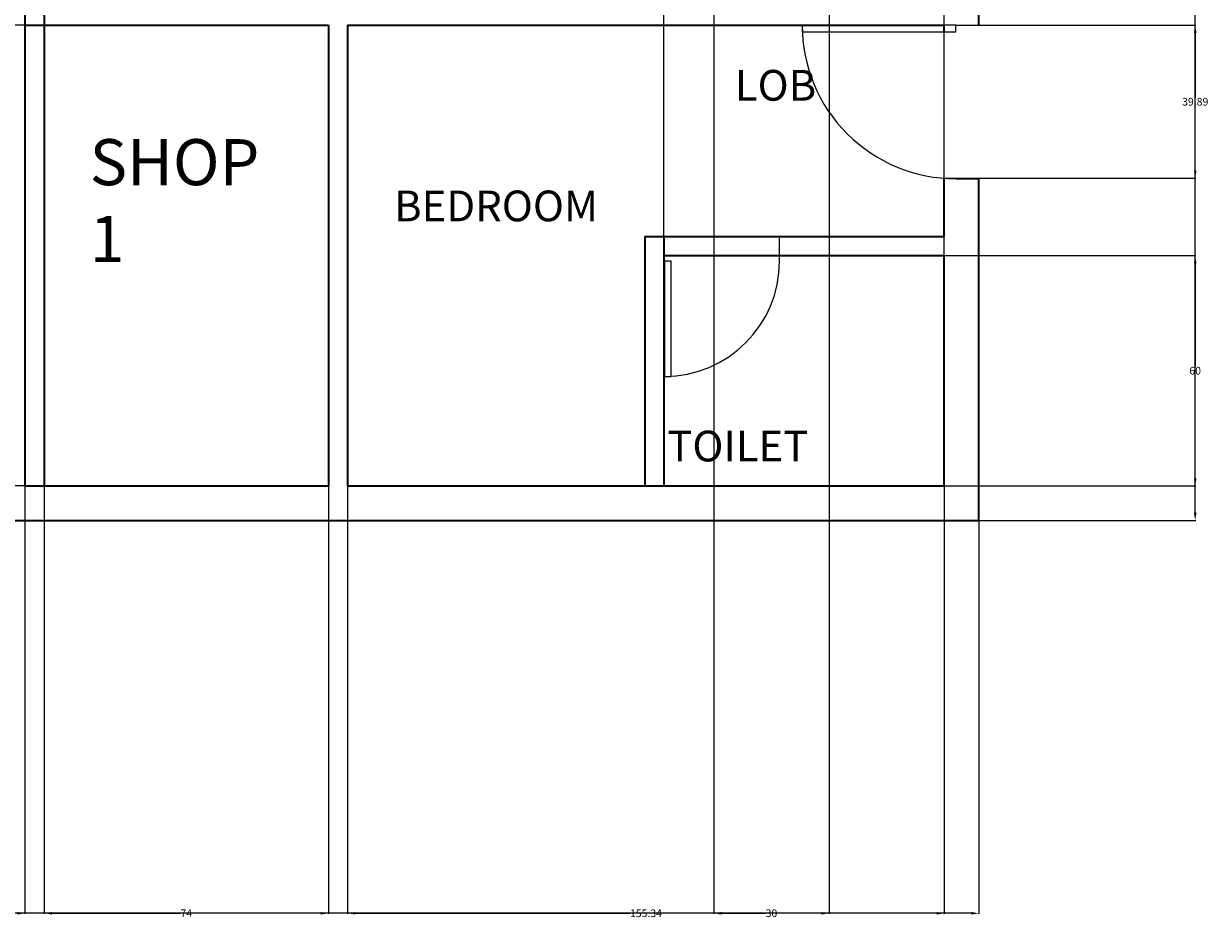
# Model space of a CAD drawing. Units: inches. Extents: x 190 to 836, y -241 to 999.
# Tile 3 of 9: x 528 to 836, y -241 to -8. Entities that reach past the tile are written whole.
import ezdxf

# ---------------------------------------------------------------- set-up
doc = ezdxf.new("R2010")
doc.units = ezdxf.units.IN
doc.header["$MEASUREMENT"] = 0
for name, color, linetype, lineweight in [('A-ANNO-DIMS', 2, 'Continuous', 18), ('A-AREA-IDEN', 7, 'Continuous', 18), ('A-DOOR', 3, 'Continuous', 18), ('A-WALL', 7, 'Continuous', 35)]:
    doc.layers.add(name, color=color, linetype=linetype, lineweight=lineweight)
doc.styles.get("Standard").update_dxf_attribs({"font": 'arial.ttf'})
doc.dimstyles.get("Standard").update_dxf_attribs({"dimtxt": 2, "dimasz": 2, "dimexe": 0.18, "dimexo": 0.0625, "dimgap": 0.09, "dimtad": 0, "dimtih": 1, "dimtoh": 1, "dimdec": 0, "dimzin": 0, "dimdsep": 46, "dimlunit": 3, "dimtxsty": 'Standard', "dimcen": 0.09, "dimadec": 0, "dimazin": 0, "dimtfac": 1, "dimtdec": 0, "dimtofl": 0, "dimtmove": 0, "dimatfit": 3, "dimfxl": 1, "dimtolj": 1, "dimtzin": 0, "dimarcsym": 0})

# ---------------------------------------------------------------- blocks, each defined once
blk = doc.blocks.new('*U3')
for p, q in [((-30, 0), (-30, -6)), ((0, 0), (0, -6))]:
    blk.add_line(p, q)
blk.add_lwpolyline([(0, 0), (0, 30), (-1.75, 30), (-1.75, 0)], close=True)
blk.add_arc((0, 0), 30, 90, 180)
blk = doc.blocks.new('*U2')
for p, q in [((0, 0), (0, 6)), ((40, 0), (40, 6))]:
    blk.add_line(p, q)
blk.add_lwpolyline([(0, 0), (0, -40), (1.75, -40), (1.75, 0)], close=True)
blk.add_arc((0, 0), 40, 270, 360)
blk = doc.blocks.new('*D16')
at = {"layer": 'A-ANNO-DIMS', "color": 0, "lineweight": -2, "transparency": 16777216}
for p, q in [((250.44, -137.53), (250.44, -239.95)), ((776.44, -137.53), (776.44, -239.95)), ((252.44, -239.77), (511.14, -239.77)), ((774.44, -239.77), (515.74, -239.77))]:
    blk.add_line(p, q, dxfattribs=at)
at = {"layer": 'A-ANNO-DIMS', "color": 0, "transparency": 16777216}
for points in [[(252.44, -239.44), (252.44, -240.11), (250.44, -239.77)], [(774.44, -239.44), (774.44, -240.11), (776.44, -239.77)]]:
    blk.add_solid(points, dxfattribs=at)
at = {"layer": 'Defpoints', "color": 0, "transparency": 16777216}
for p in [(250.44, -137.47), (776.44, -137.47), (776.44, -239.77)]:
    blk.add_point(p, dxfattribs=at)
at = {"layer": 'A-ANNO-DIMS', "color": 0, "transparency": 16777216, "insert": (513.44, -239.77), "char_height": 2, "attachment_point": 5}
blk.add_mtext('\\A1;526', dxfattribs=at)
blk = doc.blocks.new('*D18')
at = {"layer": 'A-ANNO-DIMS', "color": 0, "lineweight": -2, "transparency": 16777216}
for p, q in [((776.5, 941.53), (832.94, 941.53)), ((832.76, 939.53), (832.76, 403.14)), ((832.76, -135.47), (832.76, 400.92)), ((776.5, -137.47), (832.94, -137.47))]:
    blk.add_line(p, q, dxfattribs=at)
at = {"layer": 'A-ANNO-DIMS', "color": 0, "transparency": 16777216}
for points in [[(832.43, 939.53), (833.1, 939.53), (832.76, 941.53)], [(832.43, -135.47), (833.1, -135.47), (832.76, -137.47)]]:
    blk.add_solid(points, dxfattribs=at)
at = {"layer": 'Defpoints', "color": 0, "transparency": 16777216}
for p in [(776.44, 941.53), (832.76, 941.53), (776.44, -137.47)]:
    blk.add_point(p, dxfattribs=at)
at = {"layer": 'A-ANNO-DIMS', "color": 0, "transparency": 16777216, "insert": (832.76, 402.03), "char_height": 2, "attachment_point": 5}
blk.add_mtext('\\A1;1079', dxfattribs=at)
blk = doc.blocks.new('*D31')
at = {"layer": 'A-ANNO-DIMS', "color": 0, "lineweight": -2, "transparency": 16777216}
for p, q in [((707.44, 855.47), (707.44, -239.95)), ((737.44, 855.47), (737.44, -239.95)), ((709.44, -239.77), (720.92, -239.77)), ((735.44, -239.77), (723.96, -239.77))]:
    blk.add_line(p, q, dxfattribs=at)
at = {"layer": 'A-ANNO-DIMS', "color": 0, "transparency": 16777216}
for points in [[(709.44, -239.44), (709.44, -240.11), (707.44, -239.77)], [(735.44, -239.44), (735.44, -240.11), (737.44, -239.77)]]:
    blk.add_solid(points, dxfattribs=at)
at = {"layer": 'Defpoints', "color": 0, "transparency": 16777216}
for p in [(707.44, 855.53), (737.44, 855.53), (707.44, -239.77)]:
    blk.add_point(p, dxfattribs=at)
at = {"layer": 'A-ANNO-DIMS', "color": 0, "transparency": 16777216, "insert": (722.44, -239.77), "char_height": 2, "attachment_point": 5}
blk.add_mtext('\\A1;30', dxfattribs=at)
blk = doc.blocks.new('*D37')
at = {"layer": 'A-ANNO-DIMS', "color": 0, "lineweight": -2, "transparency": 16777216}
for p, q in [((528.1, -128.53), (528.1, -239.95)), ((447.44, -137.53), (447.44, -239.95)), ((449.44, -239.77), (484.31, -239.77)), ((526.1, -239.77), (491.24, -239.77))]:
    blk.add_line(p, q, dxfattribs=at)
at = {"layer": 'A-ANNO-DIMS', "color": 0, "transparency": 16777216}
for points in [[(449.44, -239.44), (449.44, -240.11), (447.44, -239.77)], [(526.1, -239.44), (526.1, -240.11), (528.1, -239.77)]]:
    blk.add_solid(points, dxfattribs=at)
at = {"layer": 'Defpoints', "color": 0, "transparency": 16777216}
for p in [(528.1, -128.47), (447.44, -137.47), (528.1, -239.77)]:
    blk.add_point(p, dxfattribs=at)
at = {"layer": 'A-ANNO-DIMS', "color": 0, "transparency": 16777216, "insert": (487.77, -239.77), "char_height": 2, "attachment_point": 5}
blk.add_mtext('\\A1;80.66', dxfattribs=at)
blk = doc.blocks.new('*D38')
at = {"layer": 'A-ANNO-DIMS', "color": 0, "lineweight": -2, "transparency": 16777216}
for p, q in [((533.1, -128.53), (533.1, -239.95)), ((607.1, -128.53), (607.1, -239.95)), ((535.1, -239.77), (568.59, -239.77)), ((605.1, -239.77), (571.61, -239.77))]:
    blk.add_line(p, q, dxfattribs=at)
at = {"layer": 'A-ANNO-DIMS', "color": 0, "transparency": 16777216}
for points in [[(535.1, -239.44), (535.1, -240.11), (533.1, -239.77)], [(605.1, -239.44), (605.1, -240.11), (607.1, -239.77)]]:
    blk.add_solid(points, dxfattribs=at)
at = {"layer": 'Defpoints', "color": 0, "transparency": 16777216}
for p in [(533.1, -128.47), (607.1, -128.47), (607.1, -239.77)]:
    blk.add_point(p, dxfattribs=at)
at = {"layer": 'A-ANNO-DIMS', "color": 0, "transparency": 16777216, "insert": (570.1, -239.77), "char_height": 2, "attachment_point": 5}
blk.add_mtext('\\A1;74', dxfattribs=at)
blk = doc.blocks.new('*D39')
at = {"layer": 'A-ANNO-DIMS', "color": 0, "lineweight": -2, "transparency": 16777216}
for p, q in [((612.1, -128.53), (612.1, -239.95)), ((767.44, -128.53), (767.44, -239.95)), ((614.1, -239.77), (685.63, -239.77)), ((765.44, -239.77), (693.91, -239.77))]:
    blk.add_line(p, q, dxfattribs=at)
at = {"layer": 'A-ANNO-DIMS', "color": 0, "transparency": 16777216}
for points in [[(614.1, -239.44), (614.1, -240.11), (612.1, -239.77)], [(765.44, -239.44), (765.44, -240.11), (767.44, -239.77)]]:
    blk.add_solid(points, dxfattribs=at)
at = {"layer": 'Defpoints', "color": 0, "transparency": 16777216}
for p in [(612.1, -128.47), (767.44, -128.47), (767.44, -239.77)]:
    blk.add_point(p, dxfattribs=at)
at = {"layer": 'A-ANNO-DIMS', "color": 0, "transparency": 16777216, "insert": (689.77, -239.77), "char_height": 2, "attachment_point": 5}
blk.add_mtext('\\A1;155.34', dxfattribs=at)
blk = doc.blocks.new('*D40')
at = {"layer": 'A-ANNO-DIMS', "color": 0, "lineweight": -2, "transparency": 16777216}
for p, q in [((528.04, -8.47), (193.96, -8.47)), ((194.14, -10.47), (194.14, -67.36)), ((194.14, -126.47), (194.14, -69.58)), ((533.04, -128.47), (193.96, -128.47))]:
    blk.add_line(p, q, dxfattribs=at)
at = {"layer": 'A-ANNO-DIMS', "color": 0, "transparency": 16777216}
for points in [[(193.8, -10.47), (194.47, -10.47), (194.14, -8.47)], [(193.8, -126.47), (194.47, -126.47), (194.14, -128.47)]]:
    blk.add_solid(points, dxfattribs=at)
at = {"layer": 'Defpoints', "color": 0, "transparency": 16777216}
for p in [(194.14, -8.47), (528.1, -8.47), (533.1, -128.47)]:
    blk.add_point(p, dxfattribs=at)
at = {"layer": 'A-ANNO-DIMS', "color": 0, "transparency": 16777216, "insert": (194.14, -68.47), "char_height": 2, "attachment_point": 5}
blk.add_mtext('\\A1;120', dxfattribs=at)
blk = doc.blocks.new('*D43')
at = {"layer": 'A-ANNO-DIMS', "color": 0, "lineweight": -2, "transparency": 16777216}
for p, q in [((694.44, -128.41), (694.44, 998.02)), ((696.44, 997.84), (729.43, 997.84)), ((765.44, 997.84), (732.45, 997.84)), ((767.44, -128.41), (767.44, 998.02))]:
    blk.add_line(p, q, dxfattribs=at)
at = {"layer": 'A-ANNO-DIMS', "color": 0, "transparency": 16777216}
for points in [[(696.44, 998.17), (696.44, 997.5), (694.44, 997.84)], [(765.44, 998.17), (765.44, 997.5), (767.44, 997.84)]]:
    blk.add_solid(points, dxfattribs=at)
at = {"layer": 'Defpoints', "color": 0, "transparency": 16777216}
for p in [(767.44, 997.84), (694.44, -128.47), (767.44, -128.47)]:
    blk.add_point(p, dxfattribs=at)
at = {"layer": 'A-ANNO-DIMS', "color": 0, "transparency": 16777216, "insert": (730.94, 997.84), "char_height": 2, "attachment_point": 5}
blk.add_mtext('\\A1;73', dxfattribs=at)
blk = doc.blocks.new('*D44')
at = {"layer": 'A-ANNO-DIMS', "color": 0, "lineweight": -2, "transparency": 16777216}
for p, q in [((767.5, -68.47), (832.94, -68.47)), ((832.76, -70.47), (832.76, -97.36)), ((832.76, -126.47), (832.76, -99.58)), ((767.5, -128.47), (832.94, -128.47))]:
    blk.add_line(p, q, dxfattribs=at)
at = {"layer": 'A-ANNO-DIMS', "color": 0, "transparency": 16777216}
for points in [[(832.43, -70.47), (833.1, -70.47), (832.76, -68.47)], [(832.43, -126.47), (833.1, -126.47), (832.76, -128.47)]]:
    blk.add_solid(points, dxfattribs=at)
at = {"layer": 'Defpoints', "color": 0, "transparency": 16777216}
for p in [(767.44, -68.47), (832.76, -68.47), (767.44, -128.47)]:
    blk.add_point(p, dxfattribs=at)
at = {"layer": 'A-ANNO-DIMS', "color": 0, "transparency": 16777216, "insert": (832.76, -98.47), "char_height": 2, "attachment_point": 5}
blk.add_mtext('\\A1;60', dxfattribs=at)
blk = doc.blocks.new('*D48')
at = {"layer": 'A-ANNO-DIMS', "color": 0, "lineweight": -2, "transparency": 16777216}
for p, q in [((776.5, -8.47), (832.94, -8.47)), ((832.76, -10.47), (832.76, -27.3)), ((832.76, -46.36), (832.76, -29.52)), ((767.5, -48.36), (832.94, -48.36))]:
    blk.add_line(p, q, dxfattribs=at)
at = {"layer": 'A-ANNO-DIMS', "color": 0, "transparency": 16777216}
for points in [[(832.43, -10.47), (833.1, -10.47), (832.76, -8.47)], [(832.43, -46.36), (833.1, -46.36), (832.76, -48.36)]]:
    blk.add_solid(points, dxfattribs=at)
at = {"layer": 'Defpoints', "color": 0, "transparency": 16777216}
for p in [(776.44, -8.47), (832.76, -8.47), (767.44, -48.36)]:
    blk.add_point(p, dxfattribs=at)
at = {"layer": 'A-ANNO-DIMS', "color": 0, "transparency": 16777216, "insert": (832.76, -28.41), "char_height": 2, "attachment_point": 5}
blk.add_mtext('\\A1;39.89', dxfattribs=at)

msp = doc.modelspace()

# ---------------------------------------------------------------- linework, layer by layer
at = {"layer": 'A-WALL'}
for p, q in [((776.4421, -8.4687), (776.4421, 565.5313)), ((528.0998, 115.5313), (528.0998, -128.4687)), ((533.0998, 115.5313), (533.0998, -128.4687)), ((528.0998, -8.4687), (607.0998, -8.4687)), ((607.0998, -8.4687), (607.0998, -128.4687)), ((612.0998, -8.4687), (767.4421, -8.4687)), ((612.0998, -8.4687), (612.0998, -128.4687)), ((767.4421, -10.2187), (767.4421, -8.4687)), ((767.4421, -10.2187), (767.4421, -8.4687)), ((767.4421, -63.4687), (767.4421, -48.356)), ((767.4421, -63.4687), (767.4421, -48.356)), ((776.4421, -137.4687), (776.4421, -48.4687)), ((689.4376, -63.4687), (689.4376, -128.4687)), ((689.4376, -63.4687), (767.4421, -63.4687)), ((694.4376, -68.4687), (694.4376, -128.4687)), ((694.4376, -68.4687), (767.4421, -68.4687)), ((767.4421, -128.4687), (767.4421, -68.4687)), ((767.4421, -128.4687), (767.4421, -68.4687)), ((528.0998, -128.4687), (607.0998, -128.4687)), ((528.0998, -128.4687), (607.0998, -128.4687)), ((612.0998, -128.4687), (672.0998, -128.4687)), ((612.0998, -128.4687), (767.4421, -128.4687)), ((677.0998, -128.4687), (767.4421, -128.4687)), ((499.4421, -137.4687), (776.4421, -137.4687))]:
    msp.add_line(p, q, dxfattribs=at)

# ---------------------------------------------------------------- block references
at = {"layer": 'A-DOOR'}
for name, p, rotation in [('*U2', (770.4421, -8.4687), 269.9999999999999), ('*U3', (694.5596, -69.9458), 179.9999999999999)]:
    msp.add_blockref(name, p, dxfattribs=dict(at, rotation=rotation))

# ---------------------------------------------------------------- texts
at = {"layer": 'A-AREA-IDEN'}
for s, width, insert, char_height, attachment_point in [('LOB', 33.040256, (734.1, -28.136), 8, 9), ('SHOP 1', 18.36577, (544.9435, -38.1547), 12, 1), ('BEDROOM', 33.040256, (677.2999, -59.5532), 8, 9), ('TOILET', 33.040256, (732.0386, -122.0908), 8, 9)]:
    msp.add_mtext_dynamic_manual_height_columns(s, width=width, gutter_width=1, heights=[0], dxfattribs=dict(at, insert=insert, char_height=char_height, attachment_point=attachment_point))

# ---------------------------------------------------------------- dimensions: what is measured, and where the dimension line sits
at = {"layer": 'A-ANNO-DIMS'}
for base, p1, p2, override, picture, middle in [((767.4421, 997.8363), (694.4376, -128.4687), (767.4421, -128.4687), {"dimdec": 0, "dimlfac": 1, "dimrnd": 0, "dimzin": 0, "dimdsep": 46, "dimlunit": 2}, '*D43', (730.9399, 997.8363)), ((707.4421, -239.7737), (737.4421, 855.5313), (707.4421, 855.5313), {"dimdec": 0, "dimlfac": 1, "dimrnd": 0, "dimzin": 0, "dimdsep": 46, "dimlunit": 2}, '*D31', (722.4421, -239.7737)), ((528.0998, -239.7737), (447.4421, -137.4687), (528.0998, -128.4687), {"dimdec": 2, "dimlfac": 1, "dimrnd": 0, "dimzin": 0, "dimdsep": 46, "dimlunit": 2}, '*D37', (487.771, -239.7737)), ((607.0998, -239.7737), (533.0998, -128.4687), (607.0998, -128.4687), {"dimdec": 0, "dimlfac": 1, "dimrnd": 0, "dimzin": 0, "dimdsep": 46, "dimlunit": 2}, '*D38', (570.0998, -239.7737)), ((767.4421, -239.7737), (612.0998, -128.4687), (767.4421, -128.4687), {"dimdec": 2, "dimlfac": 1, "dimrnd": 0, "dimzin": 0, "dimdsep": 46, "dimlunit": 2}, '*D39', (689.771, -239.7737)), ((776.4421, -239.7737), (250.4421, -137.4687), (776.4421, -137.4687), {"dimdec": 0, "dimlfac": 1, "dimrnd": 0, "dimzin": 0, "dimdsep": 46, "dimlunit": 2}, '*D16', (513.4421, -239.7737))]:
    dim = msp.add_linear_dim(base=base, p1=p1, p2=p2, dimstyle='Standard', override=override, dxfattribs=at)
    dim.commit()
    dim.dimension.update_dxf_attribs({"geometry": picture, "text_midpoint": middle})
for base, p1, p2, override, picture, middle in [((832.7634, 941.5313), (776.4421, -137.4687), (776.4421, 941.5313), {"dimdec": 0, "dimlfac": 1, "dimrnd": 0, "dimzin": 0, "dimdsep": 46, "dimlunit": 2}, '*D18', (832.7634, 402.0313)), ((194.1371, -8.4687), (533.0998, -128.4687), (528.0998, -8.4687), {"dimdec": 0, "dimlfac": 1, "dimrnd": 0, "dimzin": 0, "dimdsep": 46, "dimlunit": 2}, '*D40', (194.1371, -68.4687)), ((832.7634, -8.4687), (767.4421, -48.356), (776.4421, -8.4687), {"dimdec": 2, "dimlfac": 1, "dimrnd": 0, "dimzin": 0, "dimdsep": 46, "dimlunit": 2}, '*D48', (832.7634, -28.4123)), ((832.7634, -68.4687), (767.4421, -128.4687), (767.4421, -68.4687), {"dimdec": 0, "dimlfac": 1, "dimrnd": 0, "dimzin": 0, "dimdsep": 46, "dimlunit": 2}, '*D44', (832.7634, -98.4687))]:
    dim = msp.add_linear_dim(base=base, p1=p1, p2=p2, angle=90, dimstyle='Standard', override=override, dxfattribs=at)
    dim.commit()
    dim.dimension.update_dxf_attribs({"geometry": picture, "text_midpoint": middle})

doc.saveas('drawing.dxf')
